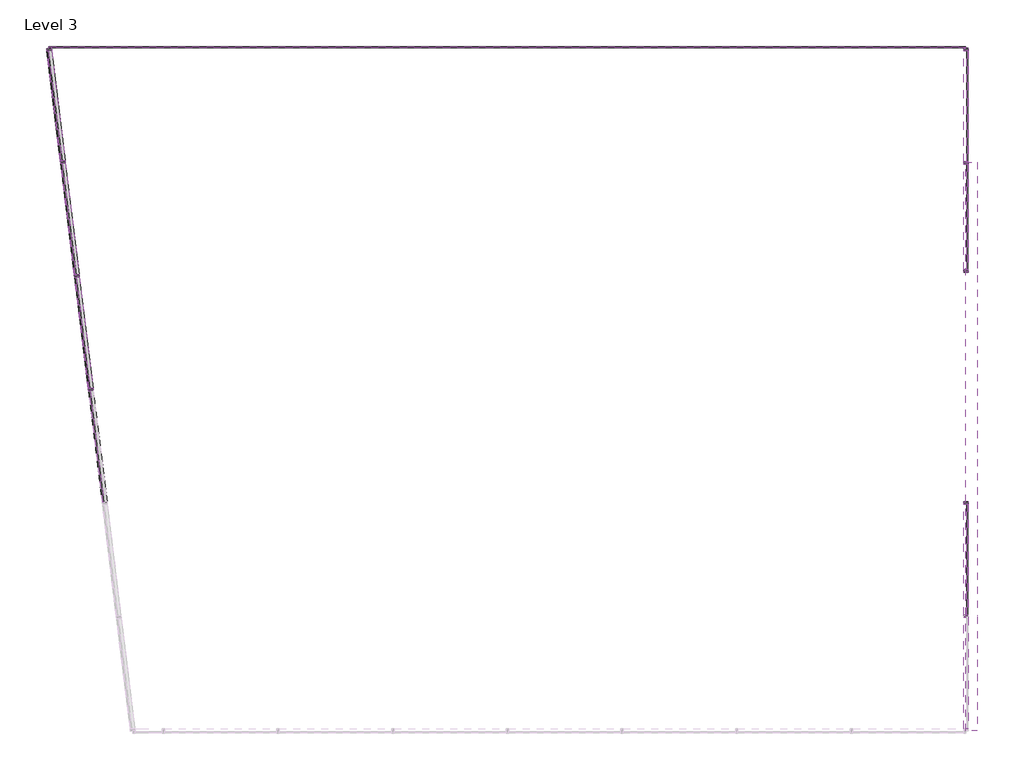
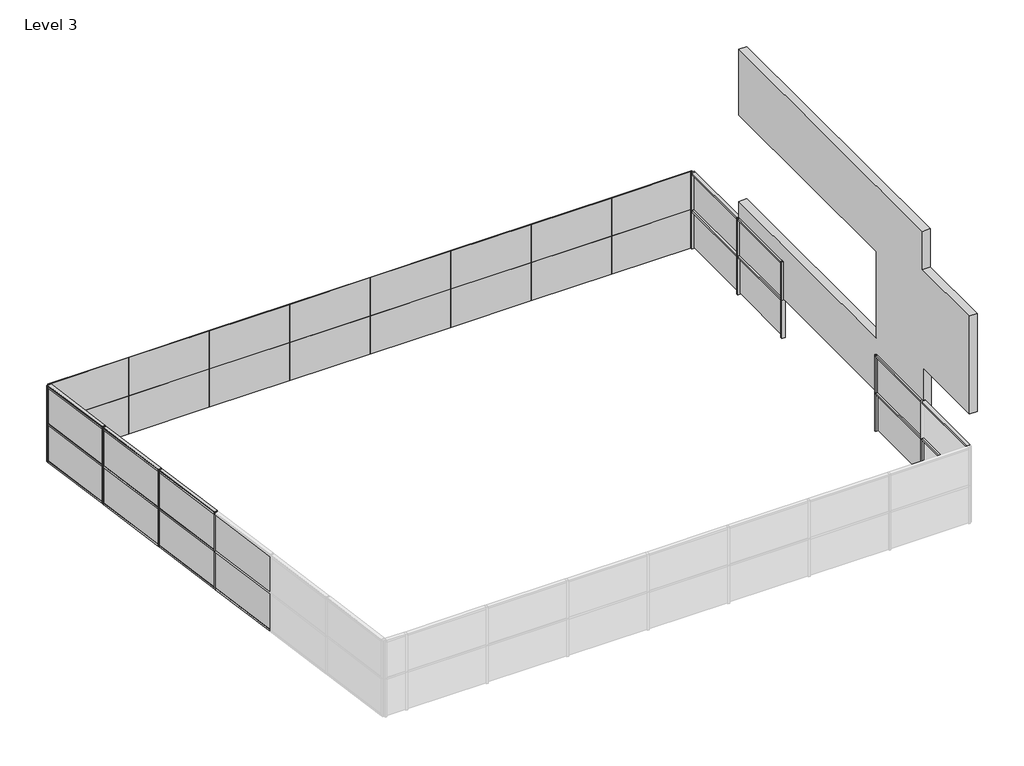
# One storey, part 2 of 2: 49 members, 38 plates, 1 proxy.
"""IFC4 building model written with IfcOpenShell, lengths in millimetres."""

from ifc_helpers import new_model, si_unit, origin, place, context, project, spatial, transform, mapped, element, save
from components import generic_models_2_generic_models_1_28cf7cb4, member_71c27fd2, member_daa7a266, member_82905deb, member_19d0a4ec, member_8cef0660, member_db480205, member_4491d118, member_46bdb8c2, member_1b94d493, system_panel_glazed_1e57f9bb, system_panel_glazed_37f15d2e, system_panel_glazed_3620f98e, system_panel_glazed_e46d4b42, system_panel_glazed_2a6c68b7, system_panel_glazed_7fb1fc2b, system_panel_glazed_d483336f

model = new_model("IFC4")

# Units and contexts
model_context = context("Model", 3, world=origin())
ifc_project = project(units=[si_unit("LENGTHUNIT", "METRE", prefix="MILLI")], contexts=[model_context])

# Site, building, storey
site = spatial("IfcSite", under=ifc_project)
building = spatial("IfcBuilding", under=site)
storey = spatial("IfcBuildingStorey", under=building, Name="Level 3", Elevation=6096.0)

# Proxy
placement = place(None, origin())
generic_models_2_generic_models_1_shape = generic_models_2_generic_models_1_28cf7cb4(model_context)
element("IfcBuildingElementProxy", 1, Name="Generic Models 2 : Generic Models 1", ObjectType="Generic Models 2 : Generic Models 1", at=placement, inside=storey, context=model_context, shape_type="MappedRepresentation", body=[
    mapped(generic_models_2_generic_models_1_shape, transform((0.0, 0.0, 8229.6), x_axis=(1.0, 0.0, 0.0), y_axis=(0.0, 1.0, 0.0), z_axis=(0.0, 0.0, 1.0))),
])

# Members
member_shape = member_71c27fd2(model_context)
element("IfcMember", 2, ObjectType="Rectangular Mullion : 2.5\" x 5\" rectangular", at=placement, inside=storey, context=model_context, shape_type="MappedRepresentation", body=[
    mapped(member_shape, transform((-10473.7456604, 11109.5209701, 6096.0), x_axis=(0.0, 0.0, -1.0), y_axis=(-0.9925461516413222, -0.12186934340514603, 0.0), z_axis=(-0.12186934340514603, 0.9925461516413222, 0.0))),
])
member_2_shape = member_daa7a266(model_context)
element("IfcMember", 3, ObjectType="Rectangular Mullion : 2.5\" x 5\" rectangular", at=placement, inside=storey, context=model_context, shape_type="MappedRepresentation", body=[
    mapped(member_2_shape, transform((-10113.8959567, 8178.7803212, 9144.0), x_axis=(0.0, 0.0, 1.0), y_axis=(-0.9925461516413222, -0.12186934340514612, 0.0), z_axis=(0.1218693434051461, -0.9925461516413221, 0.0))),
])
element("IfcMember", 4, ObjectType="Rectangular Mullion : 2.5\" x 5\" rectangular", at=placement, inside=storey, context=model_context, shape_type="MappedRepresentation", body=[
    mapped(member_2_shape, transform((13902.5156363, 11109.0476508, 9144.0), x_axis=(0.0, 0.0, 1.0), y_axis=(1.0, 0.0, 0.0), z_axis=(0.0, 1.0, 0.0))),
])
element("IfcMember", 5, ObjectType="Rectangular Mullion : 2.5\" x 5\" rectangular", at=placement, inside=storey, context=model_context, shape_type="MappedRepresentation", body=[
    mapped(member_2_shape, transform((13902.5156363, -946.6363705, 9144.0), x_axis=(0.0, 0.0, 1.0), y_axis=(1.0, 0.0, 0.0), z_axis=(0.0, 1.0, 0.0))),
])
element("IfcMember", 6, ObjectType="Rectangular Mullion : 2.5\" x 5\" rectangular", at=placement, inside=storey, context=model_context, shape_type="MappedRepresentation", body=[
    mapped(member_2_shape, transform((13902.5156363, -3962.8863708, 9144.0), x_axis=(0.0, 0.0, 1.0), y_axis=(1.0, 0.0, 0.0), z_axis=(0.0, 1.0, 0.0))),
])
member_3_shape = member_82905deb(model_context)
element("IfcMember", 7, ObjectType="Rectangular Mullion : 2.5\" x 5\" rectangular", at=placement, inside=storey, context=model_context, shape_type="MappedRepresentation", body=[
    mapped(member_3_shape, transform((-9367.1110876, 2096.7056405, 9144.0), x_axis=(-0.12186934340514591, 0.9925461516413222, 0.0), y_axis=(-0.9925461516413222, -0.12186934340514591, 0.0), z_axis=(0.0, 0.0, 1.0))),
])
element("IfcMember", 8, ObjectType="Rectangular Mullion : 2.5\" x 5\" rectangular", at=placement, inside=storey, context=model_context, shape_type="MappedRepresentation", body=[
    mapped(member_3_shape, transform((-9738.5688463, 5121.9863107, 9144.0), x_axis=(-0.12186934340514591, 0.9925461516413222, 0.0), y_axis=(-0.9925461516413222, -0.12186934340514591, 0.0), z_axis=(0.0, 0.0, 1.0))),
])
element("IfcMember", 9, ObjectType="Rectangular Mullion : 2.5\" x 5\" rectangular", at=placement, inside=storey, context=model_context, shape_type="MappedRepresentation", body=[
    mapped(member_3_shape, transform((-10110.026605, 8147.2669809, 9144.0), x_axis=(-0.12186934340514591, 0.9925461516413222, 0.0), y_axis=(-0.9925461516413222, -0.12186934340514591, 0.0), z_axis=(0.0, 0.0, 1.0))),
])
element("IfcMember", 10, ObjectType="Rectangular Mullion : 2.5\" x 5\" rectangular", at=placement, inside=storey, context=model_context, shape_type="MappedRepresentation", body=[
    mapped(member_3_shape, transform((13902.5156363, 8124.5476505, 9144.0), x_axis=(0.0, -1.0, 0.0), y_axis=(1.0, 0.0, 0.0), z_axis=(0.0, 0.0, 1.0))),
])
member_4_shape = member_19d0a4ec(model_context)
element("IfcMember", 11, ObjectType="Rectangular Mullion : 2.5\" x 5\" rectangular", at=placement, inside=storey, context=model_context, shape_type="MappedRepresentation", body=[
    mapped(member_4_shape, transform((-10113.8959567, 8178.7803212, 7620.0), x_axis=(0.0, 0.0, 1.0), y_axis=(-0.9925461516413222, -0.12186934340514603, 0.0), z_axis=(0.12186934340514602, -0.9925461516413221, 0.0))),
])
element("IfcMember", 12, ObjectType="Rectangular Mullion : 2.5\" x 5\" rectangular", at=placement, inside=storey, context=model_context, shape_type="MappedRepresentation", body=[
    mapped(member_4_shape, transform((-10113.8959567, 8178.7803212, 7620.0), x_axis=(0.0, 0.0, 1.0), y_axis=(-0.9925461516413222, -0.12186934340514603, 0.0), z_axis=(0.12186934340514603, -0.9925461516413222, 0.0))),
])
element("IfcMember", 13, ObjectType="Rectangular Mullion : 2.5\" x 5\" rectangular", at=placement, inside=storey, context=model_context, shape_type="MappedRepresentation", body=[
    mapped(member_4_shape, transform((-10113.8959567, 8178.7803212, 9144.0), x_axis=(0.0, 0.0, 1.0), y_axis=(-0.9925461516413223, -0.12186934340514535, 0.0), z_axis=(0.12186934340514535, -0.9925461516413223, 0.0))),
])
element("IfcMember", 14, ObjectType="Rectangular Mullion : 2.5\" x 5\" rectangular", at=placement, inside=storey, context=model_context, shape_type="MappedRepresentation", body=[
    mapped(member_4_shape, transform((13902.5156363, 11109.0476508, 7620.0), x_axis=(0.0, 0.0, 1.0), y_axis=(1.0, 0.0, 0.0), z_axis=(0.0, 1.0, 0.0))),
])
element("IfcMember", 15, ObjectType="Rectangular Mullion : 2.5\" x 5\" rectangular", at=placement, inside=storey, context=model_context, shape_type="MappedRepresentation", body=[
    mapped(member_4_shape, transform((13902.5156363, -946.6363705, 7620.0), x_axis=(0.0, 0.0, 1.0), y_axis=(1.0, 0.0, 0.0), z_axis=(0.0, 1.0, 0.0))),
])
element("IfcMember", 16, ObjectType="Rectangular Mullion : 2.5\" x 5\" rectangular", at=placement, inside=storey, context=model_context, shape_type="MappedRepresentation", body=[
    mapped(member_4_shape, transform((13902.5156363, -3962.8863708, 7620.0), x_axis=(0.0, 0.0, 1.0), y_axis=(1.0, 0.0, 0.0), z_axis=(0.0, 1.0, 0.0))),
])
member_5_shape = member_8cef0660(model_context)
element("IfcMember", 17, ObjectType="Rectangular Mullion : 2.5\" x 5\" rectangular", at=placement, inside=storey, context=model_context, shape_type="MappedRepresentation", body=[
    mapped(member_5_shape, transform((-9370.9804393, 2128.2189808, 7620.0), x_axis=(0.0, 0.0, 1.0), y_axis=(-0.9925461516413223, -0.12186934340514563, 0.0), z_axis=(0.12186934340514562, -0.9925461516413222, 0.0))),
])
element("IfcMember", 18, ObjectType="Rectangular Mullion : 2.5\" x 5\" rectangular", at=placement, inside=storey, context=model_context, shape_type="MappedRepresentation", body=[
    mapped(member_5_shape, transform((-9742.438198, 5153.499651, 7620.0), x_axis=(0.0, 0.0, 1.0), y_axis=(-0.9925461516413222, -0.12186934340514596, 0.0), z_axis=(0.12186934340514596, -0.9925461516413222, 0.0))),
])
element("IfcMember", 19, ObjectType="Rectangular Mullion : 2.5\" x 5\" rectangular", at=placement, inside=storey, context=model_context, shape_type="MappedRepresentation", body=[
    mapped(member_5_shape, transform((-9370.9804393, 2128.2189808, 7620.0), x_axis=(0.0, 0.0, 1.0), y_axis=(-0.9925461516413222, -0.12186934340514592, 0.0), z_axis=(0.12186934340514592, -0.9925461516413222, 0.0))),
])
element("IfcMember", 20, ObjectType="Rectangular Mullion : 2.5\" x 5\" rectangular", at=placement, inside=storey, context=model_context, shape_type="MappedRepresentation", body=[
    mapped(member_5_shape, transform((-9742.438198, 5153.499651, 7620.0), x_axis=(0.0, 0.0, 1.0), y_axis=(-0.9925461516413222, -0.12186934340514574, 0.0), z_axis=(0.12186934340514574, -0.9925461516413222, 0.0))),
])
element("IfcMember", 21, ObjectType="Rectangular Mullion : 2.5\" x 5\" rectangular", at=placement, inside=storey, context=model_context, shape_type="MappedRepresentation", body=[
    mapped(member_5_shape, transform((-9370.9804393, 2128.2189808, 9144.0), x_axis=(0.0, 0.0, 1.0), y_axis=(-0.9925461516413222, -0.12186934340514592, 0.0), z_axis=(0.12186934340514592, -0.9925461516413222, 0.0))),
])
element("IfcMember", 22, ObjectType="Rectangular Mullion : 2.5\" x 5\" rectangular", at=placement, inside=storey, context=model_context, shape_type="MappedRepresentation", body=[
    mapped(member_5_shape, transform((-9742.438198, 5153.499651, 9144.0), x_axis=(0.0, 0.0, 1.0), y_axis=(-0.9925461516413222, -0.1218693434051461, 0.0), z_axis=(0.1218693434051461, -0.9925461516413222, 0.0))),
])
member_6_shape = member_db480205(model_context)
element("IfcMember", 23, ObjectType="Rectangular Mullion : 2.5\" x 5\" rectangular", at=placement, inside=storey, context=model_context, shape_type="MappedRepresentation", body=[
    mapped(member_6_shape, transform((-9363.241736, 2065.1923001, 6096.0), x_axis=(0.0, 0.0, -1.0), y_axis=(-0.9925461516413222, -0.12186934340514602, 0.0), z_axis=(-0.12186934340514602, 0.9925461516413222, 0.0))),
])
element("IfcMember", 24, ObjectType="Rectangular Mullion : 2.5\" x 5\" rectangular", at=placement, inside=storey, context=model_context, shape_type="MappedRepresentation", body=[
    mapped(member_6_shape, transform((-9734.6994947, 5090.4729703, 6096.0), x_axis=(0.0, 0.0, -1.0), y_axis=(-0.9925461516413223, -0.12186934340514559, 0.0), z_axis=(-0.12186934340514559, 0.9925461516413223, 0.0))),
])
element("IfcMember", 25, ObjectType="Rectangular Mullion : 2.5\" x 5\" rectangular", at=placement, inside=storey, context=model_context, shape_type="MappedRepresentation", body=[
    mapped(member_6_shape, transform((-10106.1572534, 8115.7536405, 6096.0), x_axis=(0.0, 0.0, -1.0), y_axis=(-0.9925461516413222, -0.1218693434051461, 0.0), z_axis=(-0.1218693434051461, 0.9925461516413222, 0.0))),
])
element("IfcMember", 26, ObjectType="Rectangular Mullion : 2.5\" x 5\" rectangular", at=placement, inside=storey, context=model_context, shape_type="MappedRepresentation", body=[
    mapped(member_6_shape, transform((-9370.9804393, 2128.2189808, 9144.0), x_axis=(0.0, 0.0, 1.0), y_axis=(-0.9925461516413222, -0.12186934340514592, 0.0), z_axis=(0.12186934340514592, -0.9925461516413222, 0.0))),
])
element("IfcMember", 27, ObjectType="Rectangular Mullion : 2.5\" x 5\" rectangular", at=placement, inside=storey, context=model_context, shape_type="MappedRepresentation", body=[
    mapped(member_6_shape, transform((-9742.438198, 5153.499651, 9144.0), x_axis=(0.0, 0.0, 1.0), y_axis=(-0.9925461516413222, -0.12186934340514566, 0.0), z_axis=(0.12186934340514566, -0.9925461516413222, 0.0))),
])
element("IfcMember", 28, ObjectType="Rectangular Mullion : 2.5\" x 5\" rectangular", at=placement, inside=storey, context=model_context, shape_type="MappedRepresentation", body=[
    mapped(member_3_shape, transform((-9367.1110876, 2096.7056405, 7620.0), x_axis=(-0.1218693434051459, 0.9925461516413222, 0.0), y_axis=(-0.9925461516413222, -0.1218693434051459, 0.0), z_axis=(0.0, 0.0, 1.0))),
])
element("IfcMember", 29, ObjectType="Rectangular Mullion : 2.5\" x 5\" rectangular", at=placement, inside=storey, context=model_context, shape_type="MappedRepresentation", body=[
    mapped(member_3_shape, transform((-9738.5688463, 5121.9863107, 7620.0), x_axis=(-0.1218693434051459, 0.9925461516413222, 0.0), y_axis=(-0.9925461516413222, -0.1218693434051459, 0.0), z_axis=(0.0, 0.0, 1.0))),
])
element("IfcMember", 30, ObjectType="Rectangular Mullion : 2.5\" x 5\" rectangular", at=placement, inside=storey, context=model_context, shape_type="MappedRepresentation", body=[
    mapped(member_3_shape, transform((-10110.026605, 8147.2669809, 7620.0), x_axis=(-0.1218693434051459, 0.9925461516413222, 0.0), y_axis=(-0.9925461516413222, -0.1218693434051459, 0.0), z_axis=(0.0, 0.0, 1.0))),
])
element("IfcMember", 31, ObjectType="Rectangular Mullion : 2.5\" x 5\" rectangular", at=placement, inside=storey, context=model_context, shape_type="MappedRepresentation", body=[
    mapped(member_3_shape, transform((-9367.1110876, 2096.7056405, 7620.0), x_axis=(-0.12186934340514591, 0.9925461516413222, 0.0), y_axis=(-0.9925461516413222, -0.12186934340514591, 0.0), z_axis=(0.0, 0.0, 1.0))),
])
element("IfcMember", 32, ObjectType="Rectangular Mullion : 2.5\" x 5\" rectangular", at=placement, inside=storey, context=model_context, shape_type="MappedRepresentation", body=[
    mapped(member_3_shape, transform((-9738.5688463, 5121.9863107, 7620.0), x_axis=(-0.12186934340514591, 0.9925461516413222, 0.0), y_axis=(-0.9925461516413222, -0.12186934340514591, 0.0), z_axis=(0.0, 0.0, 1.0))),
])
element("IfcMember", 33, ObjectType="Rectangular Mullion : 2.5\" x 5\" rectangular", at=placement, inside=storey, context=model_context, shape_type="MappedRepresentation", body=[
    mapped(member_3_shape, transform((-10110.026605, 8147.2669809, 7620.0), x_axis=(-0.12186934340514591, 0.9925461516413222, 0.0), y_axis=(-0.9925461516413222, -0.12186934340514591, 0.0), z_axis=(0.0, 0.0, 1.0))),
])
element("IfcMember", 34, ObjectType="Rectangular Mullion : 2.5\" x 5\" rectangular", at=placement, inside=storey, context=model_context, shape_type="MappedRepresentation", body=[
    mapped(member_3_shape, transform((-9367.1110876, 2096.7056405, 9144.0), x_axis=(-0.1218693434051459, 0.9925461516413222, 0.0), y_axis=(-0.9925461516413222, -0.1218693434051459, 0.0), z_axis=(0.0, 0.0, 1.0))),
])
element("IfcMember", 35, ObjectType="Rectangular Mullion : 2.5\" x 5\" rectangular", at=placement, inside=storey, context=model_context, shape_type="MappedRepresentation", body=[
    mapped(member_3_shape, transform((-9738.5688463, 5121.9863107, 9144.0), x_axis=(-0.1218693434051459, 0.9925461516413222, 0.0), y_axis=(-0.9925461516413222, -0.1218693434051459, 0.0), z_axis=(0.0, 0.0, 1.0))),
])
element("IfcMember", 36, ObjectType="Rectangular Mullion : 2.5\" x 5\" rectangular", at=placement, inside=storey, context=model_context, shape_type="MappedRepresentation", body=[
    mapped(member_3_shape, transform((-10110.026605, 8147.2669809, 9144.0), x_axis=(-0.1218693434051459, 0.9925461516413222, 0.0), y_axis=(-0.9925461516413222, -0.1218693434051459, 0.0), z_axis=(0.0, 0.0, 1.0))),
])
element("IfcMember", 37, ObjectType="Rectangular Mullion : 2.5\" x 5\" rectangular", at=placement, inside=storey, context=model_context, shape_type="MappedRepresentation", body=[
    mapped(member_3_shape, transform((13902.5156363, 8124.5476505, 7620.0), x_axis=(0.0, -1.0, 0.0), y_axis=(1.0, 0.0, 0.0), z_axis=(0.0, 0.0, 1.0))),
])
element("IfcMember", 38, ObjectType="Rectangular Mullion : 2.5\" x 5\" rectangular", at=placement, inside=storey, context=model_context, shape_type="MappedRepresentation", body=[
    mapped(member_3_shape, transform((13902.5156363, -3931.1363708, 7620.0), x_axis=(0.0, -1.0, 0.0), y_axis=(1.0, 0.0, 0.0), z_axis=(0.0, 0.0, 1.0))),
])
member_7_shape = member_4491d118(model_context)
element("IfcMember", 39, ObjectType="Rectangular Mullion : 2.5\" x 5\" rectangular", at=placement, inside=storey, context=model_context, shape_type="MappedRepresentation", body=[
    mapped(member_7_shape, transform((-10481.4843637, 11172.5476508, 9144.0), x_axis=(-0.12186934340514591, 0.9925461516413222, 0.0), y_axis=(-0.9925461516413222, -0.12186934340514591, 0.0), z_axis=(0.0, 0.0, 1.0))),
])
element("IfcMember", 40, ObjectType="Rectangular Mullion : 2.5\" x 5\" rectangular", at=placement, inside=storey, context=model_context, shape_type="MappedRepresentation", body=[
    mapped(member_7_shape, transform((13902.5156363, 5212.8636295, 9144.0), x_axis=(0.0, -1.0, 0.0), y_axis=(1.0, 0.0, 0.0), z_axis=(0.0, 0.0, 1.0))),
])
element("IfcMember", 41, ObjectType="Rectangular Mullion : 2.5\" x 5\" rectangular", at=placement, inside=storey, context=model_context, shape_type="MappedRepresentation", body=[
    mapped(member_7_shape, transform((13902.5156363, 11172.5476508, 6096.0), x_axis=(0.0, 1.0, 0.0), y_axis=(1.0, 0.0, 0.0), z_axis=(0.0, 0.0, -1.0))),
])
element("IfcMember", 42, ObjectType="Rectangular Mullion : 2.5\" x 5\" rectangular", at=placement, inside=storey, context=model_context, shape_type="MappedRepresentation", body=[
    mapped(member_7_shape, transform((13902.5156363, -883.1363705, 6096.0), x_axis=(0.0, 1.0, 0.0), y_axis=(1.0, 0.0, 0.0), z_axis=(0.0, 0.0, -1.0))),
])
element("IfcMember", 43, ObjectType="Rectangular Mullion : 2.5\" x 5\" rectangular", at=placement, inside=storey, context=model_context, shape_type="MappedRepresentation", body=[
    mapped(member_7_shape, transform((13902.5156363, 11172.5476508, 7620.0), x_axis=(0.0, 1.0, 0.0), y_axis=(1.0, 0.0, 0.0), z_axis=(0.0, 0.0, -1.0))),
])
element("IfcMember", 44, ObjectType="Rectangular Mullion : 2.5\" x 5\" rectangular", at=placement, inside=storey, context=model_context, shape_type="MappedRepresentation", body=[
    mapped(member_7_shape, transform((13902.5156363, -883.1363705, 7620.0), x_axis=(0.0, 1.0, 0.0), y_axis=(1.0, 0.0, 0.0), z_axis=(0.0, 0.0, -1.0))),
])
element("IfcMember", 45, ObjectType="Rectangular Mullion : 2.5\" x 5\" rectangular", at=placement, inside=storey, context=model_context, shape_type="MappedRepresentation", body=[
    mapped(member_7_shape, transform((-10481.4843637, 11172.5476508, 7620.0), x_axis=(-0.1218693434051459, 0.9925461516413222, 0.0), y_axis=(-0.9925461516413222, -0.1218693434051459, 0.0), z_axis=(0.0, 0.0, 1.0))),
])
element("IfcMember", 46, ObjectType="Rectangular Mullion : 2.5\" x 5\" rectangular", at=placement, inside=storey, context=model_context, shape_type="MappedRepresentation", body=[
    mapped(member_7_shape, transform((-10481.4843637, 11172.5476508, 7620.0), x_axis=(-0.12186934340514591, 0.9925461516413222, 0.0), y_axis=(-0.9925461516413222, -0.12186934340514591, 0.0), z_axis=(0.0, 0.0, 1.0))),
])
element("IfcMember", 47, ObjectType="Rectangular Mullion : 2.5\" x 5\" rectangular", at=placement, inside=storey, context=model_context, shape_type="MappedRepresentation", body=[
    mapped(member_7_shape, transform((-10481.4843637, 11172.5476508, 9144.0), x_axis=(-0.1218693434051459, 0.9925461516413222, 0.0), y_axis=(-0.9925461516413222, -0.1218693434051459, 0.0), z_axis=(0.0, 0.0, 1.0))),
])
element("IfcMember", 48, ObjectType="Rectangular Mullion : 2.5\" x 5\" rectangular", at=placement, inside=storey, context=model_context, shape_type="MappedRepresentation", body=[
    mapped(member_7_shape, transform((13902.5156363, 5212.8636295, 7620.0), x_axis=(0.0, -1.0, 0.0), y_axis=(1.0, 0.0, 0.0), z_axis=(0.0, 0.0, 1.0))),
])
member_8_shape = member_46bdb8c2(model_context)
element("IfcMember", 49, ObjectType="Rectangular Mullion : 2.5\" x 5\" rectangular", at=placement, inside=storey, context=model_context, shape_type="MappedRepresentation", body=[
    mapped(member_8_shape, transform((13902.5156363, 8092.7976505, 7620.0), x_axis=(0.0, 0.0, 1.0), y_axis=(1.0, 0.0, 0.0), z_axis=(0.0, 1.0, 0.0))),
])
member_9_shape = member_1b94d493(model_context)
element("IfcMember", 50, ObjectType="Rectangular Mullion : 2.5\" x 5\" rectangular", at=placement, inside=storey, context=model_context, shape_type="MappedRepresentation", body=[
    mapped(member_9_shape, transform((13902.5156363, 8092.7976505, 9144.0), x_axis=(0.0, 0.0, 1.0), y_axis=(1.0, 0.0, 0.0), z_axis=(0.0, 1.0, 0.0))),
])

# Plates
system_panel_glazed_shape = system_panel_glazed_1e57f9bb(model_context)
element("IfcPlate", 51, ObjectType="System Panel : Glazed", at=placement, inside=storey, context=model_context, shape_type="MappedRepresentation", body=[
    mapped(system_panel_glazed_shape, transform((-8957.4843636, 11172.5476508, 6096.0), x_axis=(1.0, 0.0, 0.0), y_axis=(0.0, 1.0, 0.0), z_axis=(0.0, 0.0, 1.0))),
])
element("IfcPlate", 52, ObjectType="System Panel : Glazed", at=placement, inside=storey, context=model_context, shape_type="MappedRepresentation", body=[
    mapped(system_panel_glazed_shape, transform((-5909.4843634, 11172.5476508, 6096.0), x_axis=(1.0, 0.0, 0.0), y_axis=(0.0, 1.0, 0.0), z_axis=(0.0, 0.0, 1.0))),
])
element("IfcPlate", 53, ObjectType="System Panel : Glazed", at=placement, inside=storey, context=model_context, shape_type="MappedRepresentation", body=[
    mapped(system_panel_glazed_shape, transform((-2861.4843634, 11172.5476508, 6096.0), x_axis=(1.0, 0.0, 0.0), y_axis=(0.0, 1.0, 0.0), z_axis=(0.0, 0.0, 1.0))),
])
element("IfcPlate", 54, ObjectType="System Panel : Glazed", at=placement, inside=storey, context=model_context, shape_type="MappedRepresentation", body=[
    mapped(system_panel_glazed_shape, transform((186.5156366, 11172.5476508, 6096.0), x_axis=(1.0, 0.0, 0.0), y_axis=(0.0, 1.0, 0.0), z_axis=(0.0, 0.0, 1.0))),
])
element("IfcPlate", 55, ObjectType="System Panel : Glazed", at=placement, inside=storey, context=model_context, shape_type="MappedRepresentation", body=[
    mapped(system_panel_glazed_shape, transform((3234.5156366, 11172.5476508, 6096.0), x_axis=(1.0, 0.0, 0.0), y_axis=(0.0, 1.0, 0.0), z_axis=(0.0, 0.0, 1.0))),
])
element("IfcPlate", 56, ObjectType="System Panel : Glazed", at=placement, inside=storey, context=model_context, shape_type="MappedRepresentation", body=[
    mapped(system_panel_glazed_shape, transform((6282.5156366, 11172.5476508, 6096.0), x_axis=(1.0, 0.0, 0.0), y_axis=(0.0, 1.0, 0.0), z_axis=(0.0, 0.0, 1.0))),
])
element("IfcPlate", 57, ObjectType="System Panel : Glazed", at=placement, inside=storey, context=model_context, shape_type="MappedRepresentation", body=[
    mapped(system_panel_glazed_shape, transform((9330.5156366, 11172.5476508, 6096.0), x_axis=(1.0, 0.0, 0.0), y_axis=(0.0, 1.0, 0.0), z_axis=(0.0, 0.0, 1.0))),
])
element("IfcPlate", 58, ObjectType="System Panel : Glazed", at=placement, inside=storey, context=model_context, shape_type="MappedRepresentation", body=[
    mapped(system_panel_glazed_shape, transform((12378.5156364, 11172.5476508, 6096.0), x_axis=(1.0, 0.0, 0.0), y_axis=(0.0, 1.0, 0.0), z_axis=(0.0, 0.0, 1.0))),
])
element("IfcPlate", 59, ObjectType="System Panel : Glazed", at=placement, inside=storey, context=model_context, shape_type="MappedRepresentation", body=[
    mapped(system_panel_glazed_shape, transform((-8957.4843636, 11172.5476508, 7620.0), x_axis=(1.0, 0.0, 0.0), y_axis=(0.0, 1.0, 0.0), z_axis=(0.0, 0.0, 1.0))),
])
element("IfcPlate", 60, ObjectType="System Panel : Glazed", at=placement, inside=storey, context=model_context, shape_type="MappedRepresentation", body=[
    mapped(system_panel_glazed_shape, transform((-5909.4843634, 11172.5476508, 7620.0), x_axis=(1.0, 0.0, 0.0), y_axis=(0.0, 1.0, 0.0), z_axis=(0.0, 0.0, 1.0))),
])
element("IfcPlate", 61, ObjectType="System Panel : Glazed", at=placement, inside=storey, context=model_context, shape_type="MappedRepresentation", body=[
    mapped(system_panel_glazed_shape, transform((-2861.4843634, 11172.5476508, 7620.0), x_axis=(1.0, 0.0, 0.0), y_axis=(0.0, 1.0, 0.0), z_axis=(0.0, 0.0, 1.0))),
])
element("IfcPlate", 62, ObjectType="System Panel : Glazed", at=placement, inside=storey, context=model_context, shape_type="MappedRepresentation", body=[
    mapped(system_panel_glazed_shape, transform((186.5156366, 11172.5476508, 7620.0), x_axis=(1.0, 0.0, 0.0), y_axis=(0.0, 1.0, 0.0), z_axis=(0.0, 0.0, 1.0))),
])
element("IfcPlate", 63, ObjectType="System Panel : Glazed", at=placement, inside=storey, context=model_context, shape_type="MappedRepresentation", body=[
    mapped(system_panel_glazed_shape, transform((3234.5156366, 11172.5476508, 7620.0), x_axis=(1.0, 0.0, 0.0), y_axis=(0.0, 1.0, 0.0), z_axis=(0.0, 0.0, 1.0))),
])
element("IfcPlate", 64, ObjectType="System Panel : Glazed", at=placement, inside=storey, context=model_context, shape_type="MappedRepresentation", body=[
    mapped(system_panel_glazed_shape, transform((6282.5156366, 11172.5476508, 7620.0), x_axis=(1.0, 0.0, 0.0), y_axis=(0.0, 1.0, 0.0), z_axis=(0.0, 0.0, 1.0))),
])
element("IfcPlate", 65, ObjectType="System Panel : Glazed", at=placement, inside=storey, context=model_context, shape_type="MappedRepresentation", body=[
    mapped(system_panel_glazed_shape, transform((9330.5156366, 11172.5476508, 7620.0), x_axis=(1.0, 0.0, 0.0), y_axis=(0.0, 1.0, 0.0), z_axis=(0.0, 0.0, 1.0))),
])
element("IfcPlate", 66, ObjectType="System Panel : Glazed", at=placement, inside=storey, context=model_context, shape_type="MappedRepresentation", body=[
    mapped(system_panel_glazed_shape, transform((12378.5156364, 11172.5476508, 7620.0), x_axis=(1.0, 0.0, 0.0), y_axis=(0.0, 1.0, 0.0), z_axis=(0.0, 0.0, 1.0))),
])
system_panel_glazed_2_shape = system_panel_glazed_37f15d2e(model_context)
element("IfcPlate", 67, ObjectType="System Panel : Glazed", at=placement, inside=storey, context=model_context, shape_type="MappedRepresentation", body=[
    mapped(system_panel_glazed_2_shape, transform((-10293.8208085, 9644.1506457, 7651.75), x_axis=(-0.12186934340514591, 0.9925461516413222, 0.0), y_axis=(-0.9925461516413222, -0.12186934340514591, 0.0), z_axis=(0.0, 0.0, 1.0))),
])
element("IfcPlate", 68, ObjectType="System Panel : Glazed", at=placement, inside=storey, context=model_context, shape_type="MappedRepresentation", body=[
    mapped(system_panel_glazed_2_shape, transform((13902.5156363, -2423.0113706, 7651.75), x_axis=(0.0, -1.0, 0.0), y_axis=(1.0, 0.0, 0.0), z_axis=(0.0, 0.0, 1.0))),
])
element("IfcPlate", 69, ObjectType="System Panel : Glazed", at=placement, inside=storey, context=model_context, shape_type="MappedRepresentation", body=[
    mapped(system_panel_glazed_2_shape, transform((13902.5156363, 9632.6726506, 7651.75), x_axis=(0.0, -1.0, 0.0), y_axis=(1.0, 0.0, 0.0), z_axis=(0.0, 0.0, 1.0))),
])
element("IfcPlate", 70, ObjectType="System Panel : Glazed", at=placement, inside=storey, context=model_context, shape_type="MappedRepresentation", body=[
    mapped(system_panel_glazed_2_shape, transform((-10293.8208085, 9644.1506457, 6159.5), x_axis=(-0.1218693434051459, 0.9925461516413222, 0.0), y_axis=(-0.9925461516413222, -0.1218693434051459, 0.0), z_axis=(0.0, 0.0, 1.0))),
])
system_panel_glazed_3_shape = system_panel_glazed_3620f98e(model_context)
element("IfcPlate", 71, ObjectType="System Panel : Glazed", at=placement, inside=storey, context=model_context, shape_type="MappedRepresentation", body=[
    mapped(system_panel_glazed_3_shape, transform((-9181.3822083, 584.0653054, 7651.75), x_axis=(-0.12186934340514591, 0.9925461516413222, 0.0), y_axis=(-0.9925461516413222, -0.12186934340514591, 0.0), z_axis=(0.0, 0.0, 1.0))),
])
element("IfcPlate", 72, ObjectType="System Panel : Glazed", at=placement, inside=storey, context=model_context, shape_type="MappedRepresentation", body=[
    mapped(system_panel_glazed_3_shape, transform((-9552.839967, 3609.3459756, 7651.75), x_axis=(-0.12186934340514591, 0.9925461516413222, 0.0), y_axis=(-0.9925461516413222, -0.12186934340514591, 0.0), z_axis=(0.0, 0.0, 1.0))),
])
element("IfcPlate", 73, ObjectType="System Panel : Glazed", at=placement, inside=storey, context=model_context, shape_type="MappedRepresentation", body=[
    mapped(system_panel_glazed_3_shape, transform((-9924.2977257, 6634.6266458, 7651.75), x_axis=(-0.12186934340514591, 0.9925461516413222, 0.0), y_axis=(-0.9925461516413222, -0.12186934340514591, 0.0), z_axis=(0.0, 0.0, 1.0))),
])
element("IfcPlate", 74, ObjectType="System Panel : Glazed", at=placement, inside=storey, context=model_context, shape_type="MappedRepresentation", body=[
    mapped(system_panel_glazed_3_shape, transform((-9181.3822083, 584.0653054, 6159.5), x_axis=(-0.1218693434051459, 0.9925461516413222, 0.0), y_axis=(-0.9925461516413222, -0.1218693434051459, 0.0), z_axis=(0.0, 0.0, 1.0))),
])
element("IfcPlate", 75, ObjectType="System Panel : Glazed", at=placement, inside=storey, context=model_context, shape_type="MappedRepresentation", body=[
    mapped(system_panel_glazed_3_shape, transform((-9552.839967, 3609.3459756, 6159.5), x_axis=(-0.1218693434051459, 0.9925461516413222, 0.0), y_axis=(-0.9925461516413222, -0.1218693434051459, 0.0), z_axis=(0.0, 0.0, 1.0))),
])
element("IfcPlate", 76, ObjectType="System Panel : Glazed", at=placement, inside=storey, context=model_context, shape_type="MappedRepresentation", body=[
    mapped(system_panel_glazed_3_shape, transform((-9924.2977257, 6634.6266458, 6159.5), x_axis=(-0.1218693434051459, 0.9925461516413222, 0.0), y_axis=(-0.9925461516413222, -0.1218693434051459, 0.0), z_axis=(0.0, 0.0, 1.0))),
])
system_panel_glazed_4_shape = system_panel_glazed_e46d4b42(model_context)
element("IfcPlate", 77, ObjectType="System Panel : Glazed", at=placement, inside=storey, context=model_context, shape_type="MappedRepresentation", body=[
    mapped(system_panel_glazed_4_shape, transform((-10293.8208085, 9644.1506457, 6127.75), x_axis=(-0.12186934340514591, 0.9925461516413222, 0.0), y_axis=(-0.9925461516413222, -0.12186934340514591, 0.0), z_axis=(0.0, 0.0, 1.0))),
])
element("IfcPlate", 78, ObjectType="System Panel : Glazed", at=placement, inside=storey, context=model_context, shape_type="MappedRepresentation", body=[
    mapped(system_panel_glazed_4_shape, transform((13902.5156363, -2423.0113706, 6127.75), x_axis=(0.0, -1.0, 0.0), y_axis=(1.0, 0.0, 0.0), z_axis=(0.0, 0.0, 1.0))),
])
element("IfcPlate", 79, ObjectType="System Panel : Glazed", at=placement, inside=storey, context=model_context, shape_type="MappedRepresentation", body=[
    mapped(system_panel_glazed_4_shape, transform((13902.5156363, 9632.6726506, 6127.75), x_axis=(0.0, -1.0, 0.0), y_axis=(1.0, 0.0, 0.0), z_axis=(0.0, 0.0, 1.0))),
])
element("IfcPlate", 80, ObjectType="System Panel : Glazed", at=placement, inside=storey, context=model_context, shape_type="MappedRepresentation", body=[
    mapped(system_panel_glazed_4_shape, transform((-10293.8208085, 9644.1506457, 7651.75), x_axis=(-0.1218693434051459, 0.9925461516413222, 0.0), y_axis=(-0.9925461516413222, -0.1218693434051459, 0.0), z_axis=(0.0, 0.0, 1.0))),
])
system_panel_glazed_5_shape = system_panel_glazed_2a6c68b7(model_context)
element("IfcPlate", 81, ObjectType="System Panel : Glazed", at=placement, inside=storey, context=model_context, shape_type="MappedRepresentation", body=[
    mapped(system_panel_glazed_5_shape, transform((-9181.3822083, 584.0653054, 6127.75), x_axis=(-0.12186934340514591, 0.9925461516413222, 0.0), y_axis=(-0.9925461516413222, -0.12186934340514591, 0.0), z_axis=(0.0, 0.0, 1.0))),
])
element("IfcPlate", 82, ObjectType="System Panel : Glazed", at=placement, inside=storey, context=model_context, shape_type="MappedRepresentation", body=[
    mapped(system_panel_glazed_5_shape, transform((-9552.839967, 3609.3459756, 6127.75), x_axis=(-0.12186934340514591, 0.9925461516413222, 0.0), y_axis=(-0.9925461516413222, -0.12186934340514591, 0.0), z_axis=(0.0, 0.0, 1.0))),
])
element("IfcPlate", 83, ObjectType="System Panel : Glazed", at=placement, inside=storey, context=model_context, shape_type="MappedRepresentation", body=[
    mapped(system_panel_glazed_5_shape, transform((-9924.2977257, 6634.6266458, 6127.75), x_axis=(-0.12186934340514591, 0.9925461516413222, 0.0), y_axis=(-0.9925461516413222, -0.12186934340514591, 0.0), z_axis=(0.0, 0.0, 1.0))),
])
element("IfcPlate", 84, ObjectType="System Panel : Glazed", at=placement, inside=storey, context=model_context, shape_type="MappedRepresentation", body=[
    mapped(system_panel_glazed_5_shape, transform((-9181.3822083, 584.0653054, 7651.75), x_axis=(-0.1218693434051459, 0.9925461516413222, 0.0), y_axis=(-0.9925461516413222, -0.1218693434051459, 0.0), z_axis=(0.0, 0.0, 1.0))),
])
element("IfcPlate", 85, ObjectType="System Panel : Glazed", at=placement, inside=storey, context=model_context, shape_type="MappedRepresentation", body=[
    mapped(system_panel_glazed_5_shape, transform((-9552.839967, 3609.3459756, 7651.75), x_axis=(-0.1218693434051459, 0.9925461516413222, 0.0), y_axis=(-0.9925461516413222, -0.1218693434051459, 0.0), z_axis=(0.0, 0.0, 1.0))),
])
element("IfcPlate", 86, ObjectType="System Panel : Glazed", at=placement, inside=storey, context=model_context, shape_type="MappedRepresentation", body=[
    mapped(system_panel_glazed_5_shape, transform((-9924.2977257, 6634.6266458, 7651.75), x_axis=(-0.1218693434051459, 0.9925461516413222, 0.0), y_axis=(-0.9925461516413222, -0.1218693434051459, 0.0), z_axis=(0.0, 0.0, 1.0))),
])
system_panel_glazed_6_shape = system_panel_glazed_7fb1fc2b(model_context)
element("IfcPlate", 87, ObjectType="System Panel : Glazed", at=placement, inside=storey, context=model_context, shape_type="MappedRepresentation", body=[
    mapped(system_panel_glazed_6_shape, transform((13902.5156363, 6684.58064, 7651.75), x_axis=(0.0, -1.0, 0.0), y_axis=(1.0, 0.0, 0.0), z_axis=(0.0, 0.0, 1.0))),
])
system_panel_glazed_7_shape = system_panel_glazed_d483336f(model_context)
element("IfcPlate", 88, ObjectType="System Panel : Glazed", at=placement, inside=storey, context=model_context, shape_type="MappedRepresentation", body=[
    mapped(system_panel_glazed_7_shape, transform((13902.5156363, 6684.58064, 6127.75), x_axis=(0.0, -1.0, 0.0), y_axis=(1.0, 0.0, 0.0), z_axis=(0.0, 0.0, 1.0))),
])

save(model, "model.ifc")

# Revit data of these elements
# Type "Rectangular Mullion : 2.5\" x 5\" rectangular"
#   built-in parameter 1007304 = 0.416667 (stored number, unit not read)
#   built-in parameter 1007301 = 0.104167 (stored number, unit not read)
#   built-in parameter 1007300 = 0.104167 (stored number, unit not read)
# Type "System Panel : Glazed"
#   Construction Type Id = "GSP4R"
#   Analytic Construction = "1/8 in Pilkington single glazing"
#   Visual Light Transmittance = 0.9
#   Solar Heat Gain Coefficient = 0.86
#   Heat Transfer Coefficient (U) = 1.18115 BTU/(h·ft²·°F)
#   Define Thermal Properties by = 1
# Element 1 (IfcBuildingElementProxy, "Generic Models 2 : Generic Models 1")
#   Phase Created = New Construction
# Elements 2, 3, 4, 5, 6, 7, 8, 9, 10, 11, 12, 13, 14, 15, 16, 17, 18, 19, 20, 21, 22, 23, 24, 25, 26, 27, 28, 29, 30, 31, 32, 33, 34, 35, 36, 37, 38, 39, 40, 41, 42, 43, 44, 45, 46, 47, 48, 49, 50 (IfcMember, "Rectangular Mullion : 2.5\" x 5\" rectangular")
#   Phase Created = New Construction
#   Materials on its faces: "Aluminum"
# Elements 51, 52, 53, 54, 55, 56, 57, 58, 59, 60, 61, 62, 63, 64, 65, 66, 67, 68, 69, 70, 71, 72, 73, 74, 75, 76, 77, 78, 79, 80, 81, 82, 83, 84, 85, 86, 87, 88 (IfcPlate, "System Panel : Glazed")
#   Phase Created = New Construction
#   Materials on its faces: "Glass"
# Materials
#   "Aluminum": class "Metal", colour RGB 247 247 247, transparency 0, Description = "Aluminum 6061", Cost = 0
#   "Glass": class "Glass", colour RGB 0 128 192, transparency 0.75, Description = "Soda Lime Glass", Cost = 0
